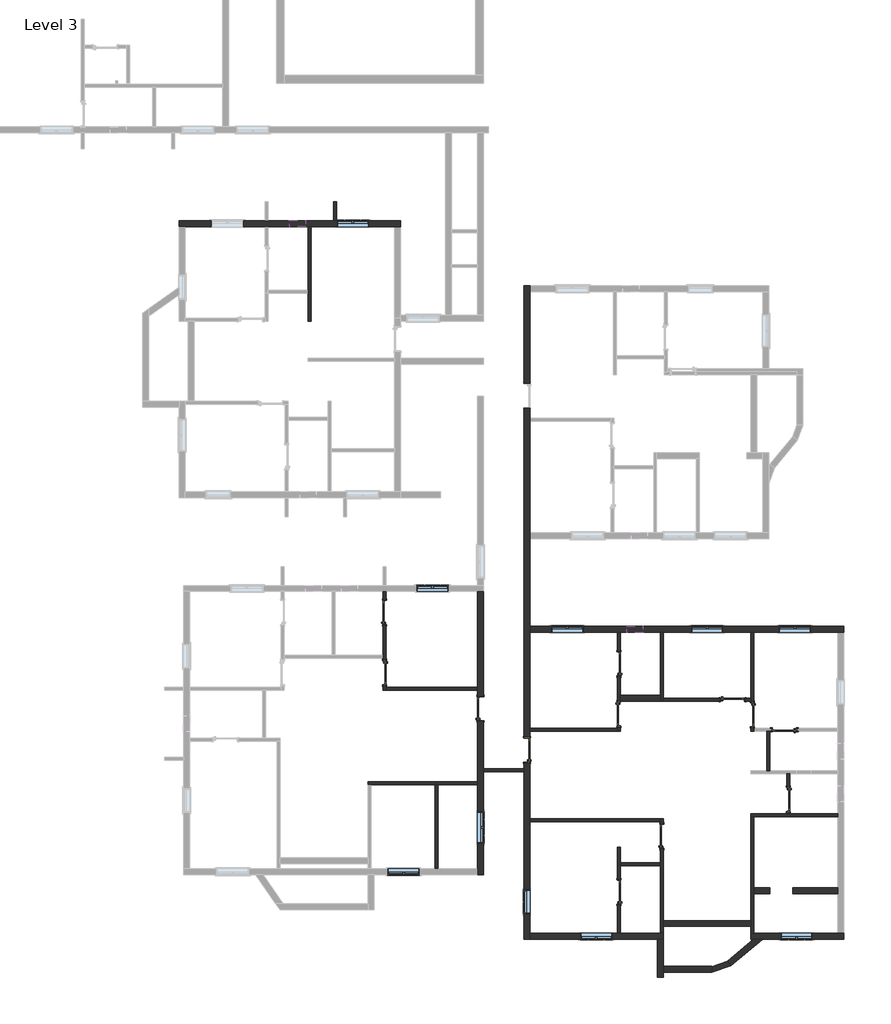
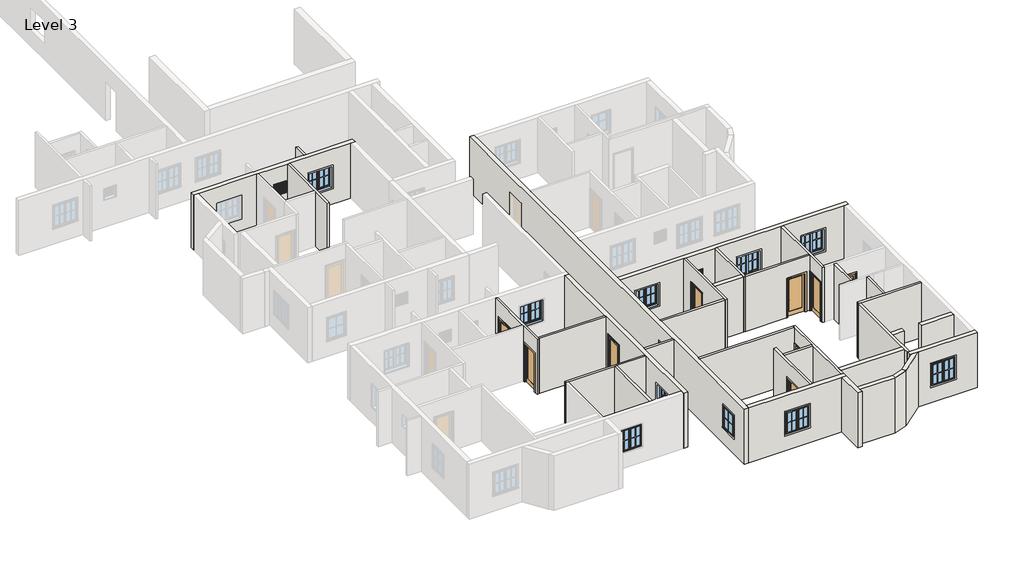
# One storey, part 2 of 7: 34 walls, 12 doors, 12 windows.
"""IFC4 building model written with IfcOpenShell, lengths in millimetres."""

from ifc_helpers import new_model, si_unit, frame, origin, place, context, project, spatial, polyline, circle_curve, outline, extrude, faceted_brep, transform, mapped, element, save
from ifc_brep_helpers import plane_surface, cylinder_surface, revolved_surface, advanced_brep
from components import door_3c6ab76a, door_a3feeac7, door_3b97b8e7, door_868ee8a9, window_272f20d6, window_casement_double_4_x_4_af3140d2, window_f2d8fef0

model = new_model("IFC4")

# Units and contexts
model_context = context("Model", 3, world=origin())
ifc_project = project(units=[si_unit("LENGTHUNIT", "METRE", prefix="MILLI")], contexts=[model_context])

# Site, building, storey
site = spatial("IfcSite", under=ifc_project)
building = spatial("IfcBuilding", under=site)
storey = spatial("IfcBuildingStorey", under=building, Name="Level 3", Elevation=3200.4)

# Doors
placement = place(None, origin())
door_shape = door_3c6ab76a(model_context)
element("IfcDoor", 1, ObjectType="Door-Interior-Single-1_Panel-Wood : 2'6\" x 7' door", at=placement, inside=storey, context=model_context, shape_type="MappedRepresentation", body=[
    mapped(door_shape, transform((13598.2490531, -20317.8247229, 3200.4), x_axis=(1.0, 0.0, 0.0), y_axis=(0.0, 1.0, 0.0), z_axis=(0.0, 0.0, 1.0))),
])
element("IfcDoor", 2, ObjectType="Door-Interior-Single-1_Panel-Wood : 2'6\" x 7' door", at=placement, inside=storey, context=model_context, shape_type="MappedRepresentation", body=[
    mapped(door_shape, transform((15579.4490531, -21467.1747229, 3200.4), x_axis=(-1.0, 0.0, 0.0), y_axis=(0.0, -1.0, 0.0), z_axis=(0.0, 0.0, 1.0))),
])
element("IfcDoor", 3, ObjectType="Door-Interior-Single-1_Panel-Wood : 2'6\" x 7' door", at=placement, inside=storey, context=model_context, shape_type="MappedRepresentation", body=[
    mapped(door_shape, transform((15735.0240531, -24130.9997229, 3200.4), x_axis=(0.0, -1.0, 0.0), y_axis=(1.0, 0.0, 0.0), z_axis=(0.0, 0.0, 1.0))),
])
element("IfcDoor", 4, ObjectType="Door-Interior-Single-1_Panel-Wood : 2'6\" x 7' door", at=placement, inside=storey, context=model_context, shape_type="MappedRepresentation", body=[
    mapped(door_shape, transform((285.4740531, -16985.9538828, 3200.4), x_axis=(0.0, 1.0, 0.0), y_axis=(-1.0, 0.0, 0.0), z_axis=(0.0, 0.0, 1.0))),
])
door_2_shape = door_a3feeac7(model_context)
element("IfcDoor", 5, ObjectType="Door-Interior-Single-1_Panel-Wood : 2'6\" x 7' door", at=placement, inside=storey, context=model_context, shape_type="MappedRepresentation", body=[
    mapped(door_2_shape, transform((9258.0240531, -18949.3997229, 3200.4), x_axis=(0.0, 1.0, 0.0), y_axis=(-1.0, 0.0, 0.0), z_axis=(0.0, 0.0, 1.0))),
])
element("IfcDoor", 6, ObjectType="Door-Interior-Single-1_Panel-Wood : 2'6\" x 7' door", at=placement, inside=storey, context=model_context, shape_type="MappedRepresentation", body=[
    mapped(door_2_shape, transform((9258.0240531, -27674.2997229, 3200.4), x_axis=(0.0, 1.0, 0.0), y_axis=(-1.0, 0.0, 0.0), z_axis=(0.0, 0.0, 1.0))),
])
element("IfcDoor", 7, ObjectType="Door-Interior-Single-1_Panel-Wood : 36\" x 84\"", at=placement, inside=storey, context=model_context, shape_type="MappedRepresentation", body=[
    mapped(door_shape, transform((14363.4240531, -20892.4997229, 3200.4), x_axis=(0.0, -1.0, 0.0), y_axis=(1.0, 0.0, 0.0), z_axis=(0.0, 0.0, 1.0))),
])
element("IfcDoor", 8, ObjectType="Door-Interior-Single-1_Panel-Wood : 36\" x 84\"", at=placement, inside=storey, context=model_context, shape_type="MappedRepresentation", body=[
    mapped(door_shape, transform((10889.9740531, -25540.6997229, 3200.4), x_axis=(0.0, 1.0, 0.0), y_axis=(-1.0, 0.0, 0.0), z_axis=(0.0, 0.0, 1.0))),
])
element("IfcDoor", 9, ObjectType="Door-Interior-Single-1_Panel-Wood : 36\" x 84\"", at=placement, inside=storey, context=model_context, shape_type="MappedRepresentation", body=[
    mapped(door_shape, transform((291.8240531, -19291.0038828, 3200.4), x_axis=(0.0, -1.0, 0.0), y_axis=(1.0, 0.0, 0.0), z_axis=(0.0, 0.0, 1.0))),
])
door_3_shape = door_3b97b8e7(model_context)
element("IfcDoor", 10, ObjectType="Door-Interior-Single-1_Panel-Wood : 36\" x 84\"", at=placement, inside=storey, context=model_context, shape_type="MappedRepresentation", body=[
    mapped(door_3_shape, transform((3962.1240531, -20662.6038828, 3200.4), x_axis=(0.0, 1.0, 0.0), y_axis=(-1.0, 0.0, 0.0), z_axis=(0.0, 0.0, 1.0))),
])
element("IfcDoor", 11, ObjectType="Door-Interior-Single-1_Panel-Wood : 36\" x 84\"", at=placement, inside=storey, context=model_context, shape_type="MappedRepresentation", body=[
    mapped(door_2_shape, transform((9251.6740531, -20863.9247229, 3200.4), x_axis=(0.0, -1.0, 0.0), y_axis=(1.0, 0.0, 0.0), z_axis=(0.0, 0.0, 1.0))),
])
door_4_shape = door_868ee8a9(model_context)
element("IfcDoor", 12, ObjectType="Door-Interior-Single-1_Panel-Wood : 36\" x 84\"", at=placement, inside=storey, context=model_context, shape_type="MappedRepresentation", body=[
    mapped(door_4_shape, transform((5733.7740531, -22245.3540434, 3200.4), x_axis=(0.0, 1.0, 0.0), y_axis=(-1.0, 0.0, 0.0), z_axis=(0.0, 0.0, 1.0))),
])

# Walls
element("IfcWall", 13, ObjectType="4.5\" wall", at=placement, inside=storey, context=model_context, shape_type="Brep", body=[
    faceted_brep([(-2524.4009469, -5860.7538828, 3200.4), (-2524.4009469, -2241.2538828, 3200.4), (-2524.4009469, -2241.2538828, 6248.4), (-2524.4009469, -5860.7538828, 6248.4), (-2638.7009469, -5860.7538828, 3200.4), (-2638.7009469, -5860.7538828, 6248.4), (-2638.7009469, -4793.9538828, 6248.4), (-2638.7009469, -4679.6538828, 6248.4), (-2638.7009469, -2241.2538828, 6248.4), (-2638.7009469, -2241.2538828, 3200.4), (-2638.7009469, -4679.6538828, 3200.4), (-2638.7009469, -4793.9538828, 3200.4)], [[[0, 1, 2, 3]], [[4, 5, 6, 7, 8, 9, 10, 11]], [[1, 0, 4, 11, 10, 9]], [[3, 2, 8, 7, 6, 5]], [[0, 3, 5, 4]], [[2, 1, 9, 8]]]),
])
element("IfcWall", 14, ObjectType="4.5\" wall", at=placement, inside=storey, context=model_context, shape_type="SweptSolid", body=[
    extrude(outline(polyline([(-1533.8009469, -1288.7538828), (-1533.8009469, -2012.6538828), (-1648.1009469, -2012.6538828), (-1648.1009469, -1288.7538828), (-1533.8009469, -1288.7538828)])), frame((0.0, 0.0, 3200.4), z_axis=(0.0, 0.0, 1.0), x_axis=(1.0, 0.0, 0.0)), (0.0, 0.0, 1.0), 3048.0),
])
element("IfcWall", 15, ObjectType="4.5\" wall", at=placement, inside=storey, context=model_context, shape_type="Brep", body=[
    faceted_brep([(345.7990531, -16185.8538828, 6248.4), (345.7990531, -19843.4538828, 6248.4), (345.7990531, -19957.7538828, 6248.4), (345.7990531, -19957.7538828, 3200.4), (345.7990531, -19843.4538828, 3200.4), (345.7990531, -19773.6038828, 3200.4), (345.7990531, -19773.6038828, 5359.4), (345.7990531, -18808.4038828, 5359.4), (345.7990531, -18808.4038828, 3200.4), (345.7990531, -17468.5538828, 3200.4), (345.7990531, -17468.5538828, 5359.4), (345.7990531, -16503.3538828, 5359.4), (345.7990531, -16503.3538828, 3200.4), (345.7990531, -16185.8538828, 3200.4), (231.4990531, -19957.7538828, 6248.4), (231.4990531, -18738.5538828, 6248.4), (231.4990531, -18624.2538828, 6248.4), (231.4990531, -16185.8538828, 6248.4), (231.4990531, -16185.8538828, 3200.4), (231.4990531, -16503.3538828, 3200.4), (231.4990531, -16503.3538828, 5359.4), (231.4990531, -17468.5538828, 5359.4), (231.4990531, -17468.5538828, 3200.4), (231.4990531, -18624.2538828, 3200.4), (231.4990531, -18738.5538828, 3200.4), (231.4990531, -18808.4038828, 3200.4), (231.4990531, -18808.4038828, 5359.4), (231.4990531, -19773.6038828, 5359.4), (231.4990531, -19773.6038828, 3200.4), (231.4990531, -19957.7538828, 3200.4)], [[[0, 1, 2, 3, 4, 5, 6, 7, 8, 9, 10, 11, 12, 13]], [[14, 15, 16, 17, 18, 19, 20, 21, 22, 23, 24, 25, 26, 27, 28, 29]], [[18, 13, 12, 19]], [[3, 29, 28, 5, 4]], [[22, 9, 8, 25, 24, 23]], [[2, 1, 0, 17, 16, 15, 14]], [[0, 13, 18, 17]], [[3, 2, 14, 29]], [[11, 20, 19, 12]], [[20, 11, 10, 21]], [[21, 10, 9, 22]], [[27, 6, 5, 28]], [[6, 27, 26, 7]], [[7, 26, 25, 8]]]),
])
element("IfcWall", 16, ObjectType="4.5\" wall", at=placement, inside=storey, context=model_context, shape_type="SweptSolid", body=[
    extrude(outline(polyline([(3850.9990531, -19957.7538828), (345.7990531, -19957.7538828), (345.7990531, -19843.4538828), (3850.9990531, -19843.4538828), (3850.9990531, -19957.7538828)])), frame((0.0, 0.0, 3200.4), z_axis=(0.0, 0.0, 1.0), x_axis=(1.0, 0.0, 0.0)), (0.0, 0.0, 1.0), 3048.0),
])
element("IfcWall", 17, ObjectType="4.5\" wall", at=placement, inside=storey, context=model_context, shape_type="Brep", body=[
    faceted_brep([(3850.9990531, -23462.9538828, 3200.4), (-340.0009469, -23462.9538828, 3200.4), (-340.0009469, -23462.9538828, 6248.4), (3850.9990531, -23462.9538828, 6248.4), (3850.9990531, -23577.2538828, 3200.4), (3850.9990531, -23577.2538828, 6248.4), (2326.9990531, -23577.2538828, 6248.4), (2212.6990531, -23577.2538828, 6248.4), (-225.7009469, -23577.2538828, 6248.4), (-340.0009469, -23577.2538828, 6248.4), (-340.0009469, -23577.2538828, 3200.4), (-225.7009469, -23577.2538828, 3200.4), (2212.6990531, -23577.2538828, 3200.4), (2326.9990531, -23577.2538828, 3200.4)], [[[0, 1, 2, 3]], [[4, 5, 6, 7, 8, 9, 10, 11, 12, 13]], [[1, 0, 4, 13, 12, 11, 10]], [[3, 2, 9, 8, 7, 6, 5]], [[0, 3, 5, 4]], [[2, 1, 10, 9]]]),
])
element("IfcWall", 18, ObjectType="4.5\" wall", at=placement, inside=storey, context=model_context, shape_type="SweptSolid", body=[
    extrude(outline(polyline([(2326.9990531, -23577.2538828), (2326.9990531, -26777.6538828), (2212.6990531, -26777.6538828), (2212.6990531, -23577.2538828), (2326.9990531, -23577.2538828)])), frame((0.0, 0.0, 3200.4), z_axis=(0.0, 0.0, 1.0), x_axis=(1.0, 0.0, 0.0)), (0.0, 0.0, 1.0), 3048.0),
])
element("IfcWall", 19, ObjectType="4.5\" wall", at=placement, inside=storey, context=model_context, shape_type="Brep", body=[
    faceted_brep([(10835.9990531, -17749.2497229, 3200.4), (10835.9990531, -20149.5497229, 3200.4), (10835.9990531, -20378.1497229, 3200.4), (10835.9990531, -20378.1497229, 6248.4), (10835.9990531, -20149.5497229, 6248.4), (10835.9990531, -17749.2497229, 6248.4), (10950.2990531, -17749.2497229, 3200.4), (10950.2990531, -17749.2497229, 6248.4), (10950.2990531, -20263.8497229, 6248.4), (10950.2990531, -20378.1497229, 6248.4), (10950.2990531, -20378.1497229, 3200.4), (10950.2990531, -20263.8497229, 3200.4)], [[[0, 1, 2, 3, 4, 5]], [[6, 7, 8, 9, 10, 11]], [[2, 1, 0, 6, 11, 10]], [[5, 4, 3, 9, 8, 7]], [[0, 5, 7, 6]], [[3, 2, 10, 9]]]),
])
element("IfcWall", 20, ObjectType="4.5\" wall", at=placement, inside=storey, context=model_context, shape_type="Brep", body=[
    faceted_brep([(9311.9990531, -17749.2497229, 6248.4), (9311.9990531, -20149.5497229, 6248.4), (9311.9990531, -20378.1497229, 6248.4), (9311.9990531, -21521.1497229, 6248.4), (9311.9990531, -21521.1497229, 3200.4), (9311.9990531, -21346.5247229, 3200.4), (9311.9990531, -21346.5247229, 5359.4), (9311.9990531, -20381.3247229, 5359.4), (9311.9990531, -20381.3247229, 3200.4), (9311.9990531, -20378.1497229, 3200.4), (9311.9990531, -20149.5497229, 3200.4), (9311.9990531, -19431.9997229, 3200.4), (9311.9990531, -19431.9997229, 5359.4), (9311.9990531, -18466.7997229, 5359.4), (9311.9990531, -18466.7997229, 3200.4), (9311.9990531, -17749.2497229, 3200.4), (9197.6990531, -21521.1497229, 6248.4), (9197.6990531, -21406.8497229, 6248.4), (9197.6990531, -17749.2497229, 6248.4), (9197.6990531, -17749.2497229, 3200.4), (9197.6990531, -18466.7997229, 3200.4), (9197.6990531, -18466.7997229, 5359.4), (9197.6990531, -19431.9997229, 5359.4), (9197.6990531, -19431.9997229, 3200.4), (9197.6990531, -20381.3247229, 3200.4), (9197.6990531, -20381.3247229, 5359.4), (9197.6990531, -21346.5247229, 5359.4), (9197.6990531, -21346.5247229, 3200.4), (9197.6990531, -21406.8497229, 3200.4), (9197.6990531, -21521.1497229, 3200.4)], [[[0, 1, 2, 3, 4, 5, 6, 7, 8, 9, 10, 11, 12, 13, 14, 15]], [[16, 17, 18, 19, 20, 21, 22, 23, 24, 25, 26, 27, 28, 29]], [[19, 15, 14, 20]], [[4, 29, 28, 27, 5]], [[8, 24, 23, 11, 10, 9]], [[3, 2, 1, 0, 18, 17, 16]], [[0, 15, 19, 18]], [[4, 3, 16, 29]], [[26, 6, 5, 27]], [[6, 26, 25, 7]], [[7, 25, 24, 8]], [[13, 21, 20, 14]], [[21, 13, 12, 22]], [[22, 12, 11, 23]]]),
])
element("IfcWall", 21, ObjectType="4.5\" wall", at=placement, inside=storey, context=model_context, shape_type="SweptSolid", body=[
    extrude(outline(polyline([(5844.8990531, -21406.8497229), (9197.6990531, -21406.8497229), (9197.6990531, -21521.1497229), (5844.8990531, -21521.1497229), (5844.8990531, -21406.8497229)])), frame((0.0, 0.0, 3200.4), z_axis=(0.0, 0.0, 1.0), x_axis=(1.0, 0.0, 0.0)), (0.0, 0.0, 1.0), 3048.0),
])
element("IfcWall", 22, ObjectType="4.5\" wall", at=placement, inside=storey, context=model_context, shape_type="Brep", body=[
    faceted_brep([(14303.0990531, -21521.1497229, 6248.4), (14303.0990531, -20378.1497229, 6248.4), (14303.0990531, -20263.8497229, 6248.4), (14303.0990531, -17749.2497229, 6248.4), (14303.0990531, -17749.2497229, 3200.4), (14303.0990531, -20263.8497229, 3200.4), (14303.0990531, -20378.1497229, 3200.4), (14303.0990531, -20409.8997229, 3200.4), (14303.0990531, -20409.8997229, 5359.4), (14303.0990531, -21375.0997229, 5359.4), (14303.0990531, -21375.0997229, 3200.4), (14303.0990531, -21521.1497229, 3200.4), (14417.3990531, -17749.2497229, 6248.4), (14417.3990531, -21406.8497229, 6248.4), (14417.3990531, -21521.1497229, 6248.4), (14417.3990531, -21521.1497229, 3200.4), (14417.3990531, -21406.8497229, 3200.4), (14417.3990531, -21375.0997229, 3200.4), (14417.3990531, -21375.0997229, 5359.4), (14417.3990531, -20409.8997229, 5359.4), (14417.3990531, -20409.8997229, 3200.4), (14417.3990531, -17749.2497229, 3200.4)], [[[0, 1, 2, 3, 4, 5, 6, 7, 8, 9, 10, 11]], [[12, 13, 14, 15, 16, 17, 18, 19, 20, 21]], [[4, 21, 20, 7, 6, 5]], [[15, 11, 10, 17, 16]], [[3, 2, 1, 0, 14, 13, 12]], [[4, 3, 12, 21]], [[0, 11, 15, 14]], [[9, 18, 17, 10]], [[18, 9, 8, 19]], [[19, 8, 7, 20]]]),
])
element("IfcWall", 23, ObjectType="4.5\" wall", at=placement, inside=storey, context=model_context, shape_type="Brep", body=[
    faceted_brep([(14303.0990531, -24797.7497229, 3200.4), (14417.3990531, -24797.7497229, 3200.4), (17617.7990531, -24797.7497229, 3200.4), (17617.7990531, -24797.7497229, 6248.4), (14417.3990531, -24797.7497229, 6248.4), (14303.0990531, -24797.7497229, 6248.4), (14303.0990531, -24683.4497229, 3200.4), (14303.0990531, -24683.4497229, 6248.4), (15674.6990531, -24683.4497229, 6248.4), (15788.9990531, -24683.4497229, 6248.4), (17617.7990531, -24683.4497229, 6248.4), (17617.7990531, -24683.4497229, 3200.4), (15788.9990531, -24683.4497229, 3200.4), (15674.6990531, -24683.4497229, 3200.4)], [[[0, 1, 2, 3, 4, 5]], [[6, 7, 8, 9, 10, 11, 12, 13]], [[2, 1, 0, 6, 13, 12, 11]], [[5, 4, 3, 10, 9, 8, 7]], [[3, 2, 11, 10]], [[0, 5, 7, 6]]]),
])
element("IfcWall", 24, ObjectType="4.5\" wall", at=placement, inside=storey, context=model_context, shape_type="Brep", body=[
    faceted_brep([(14417.3990531, -29255.4497229, 3200.4), (14417.3990531, -27731.4497229, 3200.4), (14417.3990531, -27502.8497229, 3200.4), (14417.3990531, -24797.7497229, 3200.4), (14417.3990531, -24797.7497229, 6248.4), (14417.3990531, -27502.8497229, 6248.4), (14417.3990531, -27731.4497229, 6248.4), (14417.3990531, -29255.4497229, 6248.4), (14303.0990531, -29255.4497229, 3200.4), (14303.0990531, -29255.4497229, 6248.4), (14303.0990531, -28988.7497229, 6248.4), (14303.0990531, -28760.1497229, 6248.4), (14303.0990531, -24797.7497229, 6248.4), (14303.0990531, -24797.7497229, 3200.4), (14303.0990531, -28760.1497229, 3200.4), (14303.0990531, -28988.7497229, 3200.4)], [[[0, 1, 2, 3, 4, 5, 6, 7]], [[8, 9, 10, 11, 12, 13, 14, 15]], [[3, 2, 1, 0, 8, 15, 14, 13]], [[7, 6, 5, 4, 12, 11, 10, 9]], [[4, 3, 13, 12]], [[0, 7, 9, 8]]]),
])
element("IfcWall", 25, ObjectType="4.5\" wall", at=placement, inside=storey, context=model_context, shape_type="SweptSolid", body=[
    extrude(outline(polyline([(6248.4, 14303.0990531), (6248.4, 10950.2990531), (3200.4, 10950.2990531), (3200.4, 13115.6490531), (5359.4, 13115.6490531), (5359.4, 14080.8490531), (3200.4, 14080.8490531), (3200.4, 14303.0990531), (6248.4, 14303.0990531)])), frame((0.0, -20378.1497229, 0.0), z_axis=(0.0, 1.0, 0.0), x_axis=(0.0, 0.0, 1.0)), (0.0, 0.0, 1.0), 114.3),
])
element("IfcWall", 26, ObjectType="4.5\" wall", at=placement, inside=storey, context=model_context, shape_type="SweptSolid", body=[
    extrude(outline(polyline([(14912.6990531, -23045.1497229), (14912.6990531, -21521.1497229), (15026.9990531, -21521.1497229), (15026.9990531, -23045.1497229), (14912.6990531, -23045.1497229)])), frame((0.0, 0.0, 3200.4), z_axis=(0.0, 0.0, 1.0), x_axis=(1.0, 0.0, 0.0)), (0.0, 0.0, 1.0), 3048.0),
])
element("IfcWall", 27, ObjectType="4.5\" wall", at=placement, inside=storey, context=model_context, shape_type="Brep", body=[
    faceted_brep([(10835.9990531, -29255.4497229, 6248.4), (10835.9990531, -26664.6497229, 6248.4), (10835.9990531, -26550.3497229, 6248.4), (10835.9990531, -24988.2497229, 6248.4), (10835.9990531, -24873.9497229, 6248.4), (10835.9990531, -24873.9497229, 3200.4), (10835.9990531, -24988.2497229, 3200.4), (10835.9990531, -25058.0997229, 3200.4), (10835.9990531, -25058.0997229, 5359.4), (10835.9990531, -26023.2997229, 5359.4), (10835.9990531, -26023.2997229, 3200.4), (10835.9990531, -26550.3497229, 3200.4), (10835.9990531, -26664.6497229, 3200.4), (10835.9990531, -29255.4497229, 3200.4), (10950.2990531, -24873.9497229, 6248.4), (10950.2990531, -28760.1497229, 6248.4), (10950.2990531, -28988.7497229, 6248.4), (10950.2990531, -29255.4497229, 6248.4), (10950.2990531, -29255.4497229, 3200.4), (10950.2990531, -28988.7497229, 3200.4), (10950.2990531, -28760.1497229, 3200.4), (10950.2990531, -26023.2997229, 3200.4), (10950.2990531, -26023.2997229, 5359.4), (10950.2990531, -25058.0997229, 5359.4), (10950.2990531, -25058.0997229, 3200.4), (10950.2990531, -24873.9497229, 3200.4)], [[[0, 1, 2, 3, 4, 5, 6, 7, 8, 9, 10, 11, 12, 13]], [[14, 15, 16, 17, 18, 19, 20, 21, 22, 23, 24, 25]], [[18, 13, 12, 11, 10, 21, 20, 19]], [[5, 25, 24, 7, 6]], [[4, 3, 2, 1, 0, 17, 16, 15, 14]], [[0, 13, 18, 17]], [[5, 4, 14, 25]], [[23, 8, 7, 24]], [[8, 23, 22, 9]], [[9, 22, 21, 10]]]),
])
element("IfcWall", 28, ObjectType="4.5\" wall", at=placement, inside=storey, context=model_context, shape_type="SweptSolid", body=[
    extrude(outline(polyline([(10835.9990531, -24988.2497229), (5844.8990531, -24988.2497229), (5844.8990531, -24873.9497229), (10835.9990531, -24873.9497229), (10835.9990531, -24988.2497229)])), frame((0.0, 0.0, 3200.4), z_axis=(0.0, 0.0, 1.0), x_axis=(1.0, 0.0, 0.0)), (0.0, 0.0, 1.0), 3048.0),
])
element("IfcWall", 29, ObjectType="4.5\" wall", at=placement, inside=storey, context=model_context, shape_type="SweptSolid", body=[
    extrude(outline(polyline([(-24683.4497229, 6248.4), (-23159.4497229, 6248.4), (-23159.4497229, 3200.4), (-23648.3997229, 3200.4), (-23648.3997229, 5359.4), (-24613.5997229, 5359.4), (-24613.5997229, 3200.4), (-24683.4497229, 3200.4), (-24683.4497229, 6248.4)])), frame((15674.6990531, 0.0, 0.0), z_axis=(1.0, 0.0, 0.0), x_axis=(0.0, 1.0, 0.0)), (0.0, 0.0, 1.0), 114.3),
])
element("IfcWall", 30, ObjectType="4.5\" wall", at=placement, inside=storey, context=model_context, shape_type="SweptSolid", body=[
    extrude(outline(polyline([(10835.9990531, -26664.6497229), (9311.9990531, -26664.6497229), (9311.9990531, -26550.3497229), (10835.9990531, -26550.3497229), (10835.9990531, -26664.6497229)])), frame((0.0, 0.0, 3200.4), z_axis=(0.0, 0.0, 1.0), x_axis=(1.0, 0.0, 0.0)), (0.0, 0.0, 1.0), 3048.0),
])
element("IfcWall", 31, ObjectType="4.5\" wall", at=placement, inside=storey, context=model_context, shape_type="Brep", body=[
    faceted_brep([(9311.9990531, -25953.4497229, 3200.4), (9311.9990531, -25953.4497229, 6248.4), (9311.9990531, -26550.3497229, 6248.4), (9311.9990531, -26664.6497229, 6248.4), (9311.9990531, -29255.4497229, 6248.4), (9311.9990531, -29255.4497229, 3200.4), (9311.9990531, -28156.8997229, 3200.4), (9311.9990531, -28156.8997229, 5359.4), (9311.9990531, -27191.6997229, 5359.4), (9311.9990531, -27191.6997229, 3200.4), (9311.9990531, -26664.6497229, 3200.4), (9311.9990531, -26550.3497229, 3200.4), (9197.6990531, -25953.4497229, 6248.4), (9197.6990531, -25953.4497229, 3200.4), (9197.6990531, -27191.6997229, 3200.4), (9197.6990531, -27191.6997229, 5359.4), (9197.6990531, -28156.8997229, 5359.4), (9197.6990531, -28156.8997229, 3200.4), (9197.6990531, -29255.4497229, 3200.4), (9197.6990531, -29255.4497229, 6248.4)], [[[0, 1, 2, 3, 4, 5, 6, 7, 8, 9, 10, 11]], [[12, 13, 14, 15, 16, 17, 18, 19]], [[13, 0, 11, 10, 9, 14]], [[5, 18, 17, 6]], [[1, 0, 13, 12]], [[4, 3, 2, 1, 12, 19]], [[5, 4, 19, 18]], [[8, 15, 14, 9]], [[15, 8, 7, 16]], [[16, 7, 6, 17]]]),
])
element("IfcWall", 32, ObjectType="4.5\" wall", at=placement, inside=storey, context=model_context, shape_type="SweptSolid", body=[
    extrude(outline(polyline([(4079.5990531, -22969.5583639), (5616.2990531, -22969.5583639), (5616.2990531, -23083.8583639), (4079.5990531, -23083.8583639), (4079.5990531, -22969.5583639)])), frame((0.0, 0.0, 3200.4), z_axis=(0.0, 0.0, 1.0), x_axis=(1.0, 0.0, 0.0)), (0.0, 0.0, 1.0), 3048.0),
])
element("IfcWall", 33, ObjectType="9\"", at=placement, inside=storey, context=model_context, shape_type="Brep", body=[
    faceted_brep([(904.5990531, -2012.6538828, 3200.4), (-1533.8009469, -2012.6538828, 3200.4), (-1648.1009469, -2012.6538828, 3200.4), (-4162.7009469, -2012.6538828, 3200.4), (-4277.0009469, -2012.6538828, 3200.4), (-7553.6009469, -2012.6538828, 3200.4), (-7553.6009469, -2012.6538828, 6248.4), (-4277.0009469, -2012.6538828, 6248.4), (-4162.7009469, -2012.6538828, 6248.4), (-1648.1009469, -2012.6538828, 6248.4), (-1533.8009469, -2012.6538828, 6248.4), (904.5990531, -2012.6538828, 6248.4), (-2733.9509469, -2012.6538828, 5334.0), (-3343.5509469, -2012.6538828, 5334.0), (-3343.5509469, -2012.6538828, 4724.4), (-2733.9509469, -2012.6538828, 4724.4), (-5108.8509469, -2012.6538828, 5334.0), (-6328.0509469, -2012.6538828, 5334.0), (-6328.0509469, -2012.6538828, 4114.8), (-5108.8509469, -2012.6538828, 4114.8), (-308.2509469, -2012.6538828, 5334.0), (-1527.4509469, -2012.6538828, 5334.0), (-1527.4509469, -2012.6538828, 4114.8), (-308.2509469, -2012.6538828, 4114.8), (904.5990531, -2241.2538828, 3200.4), (904.5990531, -2241.2538828, 6248.4), (675.9990531, -2241.2538828, 6248.4), (-2524.4009469, -2241.2538828, 6248.4), (-2638.7009469, -2241.2538828, 6248.4), (-4162.7009469, -2241.2538828, 6248.4), (-4277.0009469, -2241.2538828, 6248.4), (-7325.0009469, -2241.2538828, 6248.4), (-7553.6009469, -2241.2538828, 6248.4), (-7553.6009469, -2241.2538828, 3200.4), (-7325.0009469, -2241.2538828, 3200.4), (-4277.0009469, -2241.2538828, 3200.4), (-4162.7009469, -2241.2538828, 3200.4), (-2638.7009469, -2241.2538828, 3200.4), (-2524.4009469, -2241.2538828, 3200.4), (675.9990531, -2241.2538828, 3200.4), (-2733.9509469, -2241.2538828, 5334.0), (-2733.9509469, -2241.2538828, 4724.4), (-3343.5509469, -2241.2538828, 4724.4), (-3343.5509469, -2241.2538828, 5334.0), (-5108.8509469, -2241.2538828, 5334.0), (-5108.8509469, -2241.2538828, 4114.8), (-6328.0509469, -2241.2538828, 4114.8), (-6328.0509469, -2241.2538828, 5334.0), (-308.2509469, -2241.2538828, 5334.0), (-308.2509469, -2241.2538828, 4114.8), (-1527.4509469, -2241.2538828, 4114.8), (-1527.4509469, -2241.2538828, 5334.0)], [[[0, 1, 2, 3, 4, 5, 6, 7, 8, 9, 10, 11], [12, 13, 14, 15], [16, 17, 18, 19], [20, 21, 22, 23]], [[24, 25, 26, 27, 28, 29, 30, 31, 32, 33, 34, 35, 36, 37, 38, 39], [40, 41, 42, 43], [44, 45, 46, 47], [48, 49, 50, 51]], [[5, 4, 3, 2, 1, 0, 24, 39, 38, 37, 36, 35, 34, 33]], [[11, 10, 9, 8, 7, 6, 32, 31, 30, 29, 28, 27, 26, 25]], [[0, 11, 25, 24]], [[6, 5, 33, 32]], [[41, 40, 12, 15]], [[42, 41, 15, 14]], [[43, 42, 14, 13]], [[40, 43, 13, 12]], [[45, 44, 16, 19]], [[46, 45, 19, 18]], [[47, 46, 18, 17]], [[44, 47, 17, 16]], [[49, 48, 20, 23]], [[50, 49, 23, 22]], [[51, 50, 22, 21]], [[48, 51, 21, 20]]]),
])
element("IfcWall", 34, ObjectType="9\"", at=placement, inside=storey, context=model_context, shape_type="Brep", body=[
    faceted_brep([(4079.5990531, -16185.8538828, 6248.4), (4079.5990531, -22969.5583639, 6248.4), (4079.5990531, -23083.8583639, 6248.4), (4079.5990531, -27006.2538828, 6248.4), (4079.5990531, -27006.2538828, 3200.4), (4079.5990531, -23083.8583639, 3200.4), (4079.5990531, -22969.5583639, 3200.4), (4079.5990531, -21145.2038828, 3200.4), (4079.5990531, -21145.2038828, 5359.4), (4079.5990531, -20180.0038828, 5359.4), (4079.5990531, -20180.0038828, 3200.4), (4079.5990531, -16185.8538828, 3200.4), (4079.5990531, -25815.6288828, 5334.0), (4079.5990531, -24596.4288828, 5334.0), (4079.5990531, -24596.4288828, 4114.8), (4079.5990531, -25815.6288828, 4114.8), (3850.9990531, -27006.2538828, 6248.4), (3850.9990531, -26777.6538828, 6248.4), (3850.9990531, -23577.2538828, 6248.4), (3850.9990531, -23462.9538828, 6248.4), (3850.9990531, -19957.7538828, 6248.4), (3850.9990531, -19843.4538828, 6248.4), (3850.9990531, -16185.8538828, 6248.4), (3850.9990531, -16185.8538828, 3200.4), (3850.9990531, -19843.4538828, 3200.4), (3850.9990531, -19957.7538828, 3200.4), (3850.9990531, -20180.0038828, 3200.4), (3850.9990531, -20180.0038828, 5359.4), (3850.9990531, -21145.2038828, 5359.4), (3850.9990531, -21145.2038828, 3200.4), (3850.9990531, -23462.9538828, 3200.4), (3850.9990531, -23577.2538828, 3200.4), (3850.9990531, -26777.6538828, 3200.4), (3850.9990531, -27006.2538828, 3200.4), (3850.9990531, -25815.6288828, 5334.0), (3850.9990531, -25815.6288828, 4114.8), (3850.9990531, -24596.4288828, 4114.8), (3850.9990531, -24596.4288828, 5334.0)], [[[0, 1, 2, 3, 4, 5, 6, 7, 8, 9, 10, 11], [12, 13, 14, 15]], [[16, 17, 18, 19, 20, 21, 22, 23, 24, 25, 26, 27, 28, 29, 30, 31, 32, 33], [34, 35, 36, 37]], [[4, 33, 32, 31, 30, 29, 7, 6, 5]], [[23, 11, 10, 26, 25, 24]], [[3, 2, 1, 0, 22, 21, 20, 19, 18, 17, 16]], [[4, 3, 16, 33]], [[0, 11, 23, 22]], [[9, 27, 26, 10]], [[27, 9, 8, 28]], [[28, 8, 7, 29]], [[35, 34, 12, 15]], [[36, 35, 15, 14]], [[37, 36, 14, 13]], [[34, 37, 13, 12]]]),
])
element("IfcWall", 35, ObjectType="9\"", at=placement, inside=storey, context=model_context, shape_type="Brep", body=[
    faceted_brep([(5844.8990531, -17749.2497229, 3200.4), (9197.6990531, -17749.2497229, 3200.4), (9311.9990531, -17749.2497229, 3200.4), (10835.9990531, -17749.2497229, 3200.4), (10950.2990531, -17749.2497229, 3200.4), (14303.0990531, -17749.2497229, 3200.4), (14417.3990531, -17749.2497229, 3200.4), (17617.7990531, -17749.2497229, 3200.4), (17846.3990531, -17749.2497229, 3200.4), (17846.3990531, -17749.2497229, 6248.4), (17617.7990531, -17749.2497229, 6248.4), (14417.3990531, -17749.2497229, 6248.4), (14303.0990531, -17749.2497229, 6248.4), (10950.2990531, -17749.2497229, 6248.4), (10835.9990531, -17749.2497229, 6248.4), (9311.9990531, -17749.2497229, 6248.4), (9197.6990531, -17749.2497229, 6248.4), (5844.8990531, -17749.2497229, 6248.4), (10169.2490531, -17749.2497229, 5334.0), (10169.2490531, -17749.2497229, 4724.4), (9559.6490531, -17749.2497229, 4724.4), (9559.6490531, -17749.2497229, 5334.0), (7889.5990531, -17749.2497229, 5334.0), (7889.5990531, -17749.2497229, 4114.8), (6670.3990531, -17749.2497229, 4114.8), (6670.3990531, -17749.2497229, 5334.0), (13236.2990531, -17749.2497229, 5334.0), (13236.2990531, -17749.2497229, 4114.8), (12017.0990531, -17749.2497229, 4114.8), (12017.0990531, -17749.2497229, 5334.0), (16595.4490531, -17749.2497229, 5334.0), (16595.4490531, -17749.2497229, 4114.8), (15376.2490531, -17749.2497229, 4114.8), (15376.2490531, -17749.2497229, 5334.0), (5844.8990531, -17520.6497229, 3200.4), (5844.8990531, -17520.6497229, 6248.4), (17846.3990531, -17520.6497229, 6248.4), (17846.3990531, -17520.6497229, 3200.4), (10169.2490531, -17520.6497229, 5334.0), (9559.6490531, -17520.6497229, 5334.0), (9559.6490531, -17520.6497229, 4724.4), (10169.2490531, -17520.6497229, 4724.4), (7889.5990531, -17520.6497229, 5334.0), (6670.3990531, -17520.6497229, 5334.0), (6670.3990531, -17520.6497229, 4114.8), (7889.5990531, -17520.6497229, 4114.8), (13236.2990531, -17520.6497229, 5334.0), (12017.0990531, -17520.6497229, 5334.0), (12017.0990531, -17520.6497229, 4114.8), (13236.2990531, -17520.6497229, 4114.8), (16595.4490531, -17520.6497229, 5334.0), (15376.2490531, -17520.6497229, 5334.0), (15376.2490531, -17520.6497229, 4114.8), (16595.4490531, -17520.6497229, 4114.8)], [[[0, 1, 2, 3, 4, 5, 6, 7, 8, 9, 10, 11, 12, 13, 14, 15, 16, 17], [18, 19, 20, 21], [22, 23, 24, 25], [26, 27, 28, 29], [30, 31, 32, 33]], [[34, 35, 36, 37], [38, 39, 40, 41], [42, 43, 44, 45], [46, 47, 48, 49], [50, 51, 52, 53]], [[8, 7, 6, 5, 4, 3, 2, 1, 0, 34, 37]], [[17, 16, 15, 14, 13, 12, 11, 10, 9, 36, 35]], [[0, 17, 35, 34]], [[9, 8, 37, 36]], [[19, 18, 38, 41]], [[20, 19, 41, 40]], [[21, 20, 40, 39]], [[18, 21, 39, 38]], [[23, 22, 42, 45]], [[24, 23, 45, 44]], [[25, 24, 44, 43]], [[22, 25, 43, 42]], [[27, 26, 46, 49]], [[28, 27, 49, 48]], [[29, 28, 48, 47]], [[26, 29, 47, 46]], [[31, 30, 50, 53]], [[32, 31, 53, 52]], [[33, 32, 52, 51]], [[30, 33, 51, 50]]]),
])
element("IfcWall", 36, ObjectType="9\"", at=placement, inside=storey, context=model_context, shape_type="Brep", body=[
    faceted_brep([(5844.8990531, -4503.1497229, 6248.4), (5844.8990531, -4731.7497229, 6248.4), (5844.8990531, -9557.7497229, 6248.4), (5844.8990531, -9672.0497229, 6248.4), (5844.8990531, -13939.2497229, 6248.4), (5844.8990531, -14167.8497229, 6248.4), (5844.8990531, -17520.6497229, 6248.4), (5844.8990531, -17749.2497229, 6248.4), (5844.8990531, -21406.8497229, 6248.4), (5844.8990531, -21521.1497229, 6248.4), (5844.8990531, -24873.9497229, 6248.4), (5844.8990531, -24988.2497229, 6248.4), (5844.8990531, -29255.4497229, 6248.4), (5844.8990531, -29484.0497229, 6248.4), (5844.8990531, -29484.0497229, 3200.4), (5844.8990531, -29255.4497229, 3200.4), (5844.8990531, -24988.2497229, 3200.4), (5844.8990531, -24873.9497229, 3200.4), (5844.8990531, -22727.9540434, 3200.4), (5844.8990531, -22727.9540434, 5359.4), (5844.8990531, -21762.7540434, 5359.4), (5844.8990531, -21762.7540434, 3200.4), (5844.8990531, -21521.1497229, 3200.4), (5844.8990531, -21406.8497229, 3200.4), (5844.8990531, -17749.2497229, 3200.4), (5844.8990531, -17520.6497229, 3200.4), (5844.8990531, -14167.8497229, 3200.4), (5844.8990531, -13939.2497229, 3200.4), (5844.8990531, -9672.0497229, 3200.4), (5844.8990531, -9557.7497229, 3200.4), (5844.8990531, -9183.0997229, 3200.4), (5844.8990531, -9183.0997229, 5359.4), (5844.8990531, -8217.8997229, 5359.4), (5844.8990531, -8217.8997229, 3200.4), (5844.8990531, -4731.7497229, 3200.4), (5844.8990531, -4503.1497229, 3200.4), (5844.8990531, -27591.7497229, 5334.0), (5844.8990531, -27591.7497229, 4114.8), (5844.8990531, -28506.1497229, 4114.8), (5844.8990531, -28506.1497229, 5334.0), (5616.2990531, -29484.0497229, 6248.4), (5616.2990531, -23083.8583639, 6248.4), (5616.2990531, -22969.5583639, 6248.4), (5616.2990531, -4503.1497229, 6248.4), (5616.2990531, -4503.1497229, 3200.4), (5616.2990531, -8217.8997229, 3200.4), (5616.2990531, -8217.8997229, 5359.4), (5616.2990531, -9183.0997229, 5359.4), (5616.2990531, -9183.0997229, 3200.4), (5616.2990531, -21762.7540434, 3200.4), (5616.2990531, -21762.7540434, 5359.4), (5616.2990531, -22727.9540434, 5359.4), (5616.2990531, -22727.9540434, 3200.4), (5616.2990531, -22969.5583639, 3200.4), (5616.2990531, -23083.8583639, 3200.4), (5616.2990531, -29484.0497229, 3200.4), (5616.2990531, -27591.7497229, 5334.0), (5616.2990531, -28506.1497229, 5334.0), (5616.2990531, -28506.1497229, 4114.8), (5616.2990531, -27591.7497229, 4114.8)], [[[0, 1, 2, 3, 4, 5, 6, 7, 8, 9, 10, 11, 12, 13, 14, 15, 16, 17, 18, 19, 20, 21, 22, 23, 24, 25, 26, 27, 28, 29, 30, 31, 32, 33, 34, 35], [36, 37, 38, 39]], [[40, 41, 42, 43, 44, 45, 46, 47, 48, 49, 50, 51, 52, 53, 54, 55], [56, 57, 58, 59]], [[14, 55, 54, 53, 52, 18, 17, 16, 15]], [[44, 35, 34, 33, 45]], [[48, 30, 29, 28, 27, 26, 25, 24, 23, 22, 21, 49]], [[13, 12, 11, 10, 9, 8, 7, 6, 5, 4, 3, 2, 1, 0, 43, 42, 41, 40]], [[14, 13, 40, 55]], [[0, 35, 44, 43]], [[47, 31, 30, 48]], [[31, 47, 46, 32]], [[32, 46, 45, 33]], [[20, 50, 49, 21]], [[50, 20, 19, 51]], [[51, 19, 18, 52]], [[37, 36, 56, 59]], [[38, 37, 59, 58]], [[39, 38, 58, 57]], [[36, 39, 57, 56]]]),
])
element("IfcWall", 37, ObjectType="9\"", at=placement, inside=storey, context=model_context, shape_type="Brep", body=[
    faceted_brep([(5844.8990531, -29484.0497229, 3200.4), (10721.6990531, -29484.0497229, 3200.4), (10950.2990531, -29484.0497229, 3200.4), (10950.2990531, -29484.0497229, 6248.4), (10721.6990531, -29484.0497229, 6248.4), (5844.8990531, -29484.0497229, 6248.4), (7781.6490531, -29484.0497229, 5334.0), (9000.8490531, -29484.0497229, 5334.0), (9000.8490531, -29484.0497229, 4114.8), (7781.6490531, -29484.0497229, 4114.8), (5844.8990531, -29255.4497229, 3200.4), (5844.8990531, -29255.4497229, 6248.4), (9197.6990531, -29255.4497229, 6248.4), (9311.9990531, -29255.4497229, 6248.4), (10835.9990531, -29255.4497229, 6248.4), (10950.2990531, -29255.4497229, 6248.4), (10950.2990531, -29255.4497229, 3200.4), (10835.9990531, -29255.4497229, 3200.4), (9311.9990531, -29255.4497229, 3200.4), (9197.6990531, -29255.4497229, 3200.4), (7781.6490531, -29255.4497229, 5334.0), (7781.6490531, -29255.4497229, 4114.8), (9000.8490531, -29255.4497229, 4114.8), (9000.8490531, -29255.4497229, 5334.0)], [[[0, 1, 2, 3, 4, 5], [6, 7, 8, 9]], [[10, 11, 12, 13, 14, 15, 16, 17, 18, 19], [20, 21, 22, 23]], [[2, 1, 0, 10, 19, 18, 17, 16]], [[5, 4, 3, 15, 14, 13, 12, 11]], [[0, 5, 11, 10]], [[3, 2, 16, 15]], [[21, 20, 6, 9]], [[22, 21, 9, 8]], [[23, 22, 8, 7]], [[20, 23, 7, 6]]]),
])
element("IfcWall", 38, ObjectType="9\"", at=placement, inside=storey, context=model_context, shape_type="SweptSolid", body=[
    extrude(outline(polyline([(9311.9990531, -20149.5497229), (10835.9990531, -20149.5497229), (10835.9990531, -20378.1497229), (9311.9990531, -20378.1497229), (9311.9990531, -20149.5497229)])), frame((0.0, 0.0, 3200.4), z_axis=(0.0, 0.0, 1.0), x_axis=(1.0, 0.0, 0.0)), (0.0, 0.0, 1.0), 3048.0),
])
element("IfcWall", 39, ObjectType="9\"", at=placement, inside=storey, context=model_context, shape_type="SweptSolid", body=[
    extrude(outline(polyline([(17617.7990531, -27731.4497229), (15901.9350228, -27731.4497229), (15901.9350228, -27502.8497229), (17617.7990531, -27502.8497229), (17617.7990531, -27731.4497229)])), frame((0.0, 0.0, 3200.4), z_axis=(0.0, 0.0, 1.0), x_axis=(1.0, 0.0, 0.0)), (0.0, 0.0, 1.0), 3048.0),
])
element("IfcWall", 40, ObjectType="9\"", at=placement, inside=storey, context=model_context, shape_type="SweptSolid", body=[
    extrude(outline(polyline([(15026.9990531, -27731.4497229), (14417.3990531, -27731.4497229), (14417.3990531, -27502.8497229), (15026.9990531, -27502.8497229), (15026.9990531, -27731.4497229)])), frame((0.0, 0.0, 3200.4), z_axis=(0.0, 0.0, 1.0), x_axis=(1.0, 0.0, 0.0)), (0.0, 0.0, 1.0), 3048.0),
])
element("IfcWall", 41, ObjectType="9\"", at=placement, inside=storey, context=model_context, shape_type="SweptSolid", body=[
    extrude(outline(polyline([(14303.0990531, -28988.7497229), (10950.2990531, -28988.7497229), (10950.2990531, -28760.1497229), (14303.0990531, -28760.1497229), (14303.0990531, -28988.7497229)])), frame((0.0, 0.0, 3200.4), z_axis=(0.0, 0.0, 1.0), x_axis=(1.0, 0.0, 0.0)), (0.0, 0.0, 1.0), 3048.0),
])
element("IfcWall", 42, ObjectType="9\"", at=placement, inside=storey, context=model_context, shape_type="Brep", body=[
    faceted_brep([(14303.0990531, -29484.0497229, 3200.4), (14391.7049387, -29484.0497229, 3200.4), (14750.9761043, -29484.0497229, 3200.4), (17846.3990531, -29484.0497229, 3200.4), (17846.3990531, -29484.0497229, 6248.4), (14750.9761043, -29484.0497229, 6248.4), (14391.7049387, -29484.0497229, 6248.4), (14303.0990531, -29484.0497229, 6248.4), (15436.5740531, -29484.0497229, 5334.0), (16655.7740531, -29484.0497229, 5334.0), (16655.7740531, -29484.0497229, 4114.8), (15436.5740531, -29484.0497229, 4114.8), (14303.0990531, -29255.4497229, 3200.4), (14303.0990531, -29255.4497229, 6248.4), (14417.3990531, -29255.4497229, 6248.4), (17617.7990531, -29255.4497229, 6248.4), (17846.3990531, -29255.4497229, 6248.4), (17846.3990531, -29255.4497229, 3200.4), (17617.7990531, -29255.4497229, 3200.4), (14417.3990531, -29255.4497229, 3200.4), (15436.5740531, -29255.4497229, 5334.0), (15436.5740531, -29255.4497229, 4114.8), (16655.7740531, -29255.4497229, 4114.8), (16655.7740531, -29255.4497229, 5334.0)], [[[0, 1, 2, 3, 4, 5, 6, 7], [8, 9, 10, 11]], [[12, 13, 14, 15, 16, 17, 18, 19], [20, 21, 22, 23]], [[3, 2, 1, 0, 12, 19, 18, 17]], [[7, 6, 5, 4, 16, 15, 14, 13]], [[4, 3, 17, 16]], [[0, 7, 13, 12]], [[21, 20, 8, 11]], [[22, 21, 11, 10]], [[23, 22, 10, 9]], [[20, 23, 9, 8]]]),
])
element("IfcWall", 43, ObjectType="9\"", at=placement, inside=storey, context=model_context, shape_type="Brep", body=[
    faceted_brep([(10950.2990531, -30936.1779934, 3200.4), (10950.2990531, -30741.3497229, 3200.4), (10950.2990531, -30512.7497229, 3200.4), (10950.2990531, -29484.0497229, 3200.4), (10950.2990531, -29484.0497229, 6248.4), (10950.2990531, -30512.7497229, 6248.4), (10950.2990531, -30741.3497229, 6248.4), (10950.2990531, -30936.1779934, 6248.4), (10721.6990531, -30936.1779934, 3200.4), (10721.6990531, -30936.1779934, 6248.4), (10721.6990531, -29484.0497229, 6248.4), (10721.6990531, -29484.0497229, 3200.4)], [[[0, 1, 2, 3, 4, 5, 6, 7]], [[8, 9, 10, 11]], [[3, 2, 1, 0, 8, 11]], [[7, 6, 5, 4, 10, 9]], [[0, 7, 9, 8]], [[4, 3, 11, 10]]]),
])
element("IfcWall", 44, ObjectType="9\"", at=placement, inside=storey, context=model_context, shape_type="Brep", body=[
    faceted_brep([(12809.2934887, -30512.7497229, 3200.4), (10950.2990531, -30512.7497229, 3200.4), (10950.2990531, -30512.7497229, 6248.4), (12809.2934887, -30512.7497229, 6248.4), (12809.2934887, -30741.3497229, 3200.4), (12809.2934887, -30741.3497229, 6248.4), (10950.2990531, -30741.3497229, 6248.4), (10950.2990531, -30741.3497229, 3200.4), (12809.2934887, -30518.3143222, 3200.4), (12809.2934887, -30518.3143222, 6248.4)], [[[0, 1, 2, 3]], [[4, 5, 6, 7]], [[1, 0, 8, 4, 7]], [[3, 2, 6, 5, 9]], [[0, 3, 9, 5, 4, 8]], [[2, 1, 7, 6]]]),
])
element("IfcWall", 45, ObjectType="9\"", at=placement, inside=storey, context=model_context, shape_type="AdvancedBrep", body=[
    advanced_brep(
    [(13391.1154104, -30309.3295271, 6248.4), (12809.2934887, -30518.3143222, 6248.4), (12809.2934887, -30741.3497229, 6248.4), (12809.2934887, -30746.9143222, 6248.4), (13536.5708908, -30485.6833283, 6248.4), (13391.1154104, -30309.3295271, 3200.4), (13536.5708908, -30485.6833283, 3200.4), (12809.2934887, -30746.9143222, 3200.4), (12809.2934887, -30741.3497229, 3200.4), (12809.2934887, -30518.3143222, 3200.4)],
    [
        (0, 1, circle_curve(frame((12809.2934887, -29603.9143222, 6248.4), z_axis=(0.0, 0.0, -1.0), x_axis=(0.0, -1.0, 0.0)), 914.4)),
        (1, 2),
        (2, 3),
        (3, 4, circle_curve(frame((12809.2934887, -29603.9143222, 6248.4), z_axis=(0.0, 0.0, 1.0), x_axis=(0.0, -1.0, 0.0)), 1143.0)),
        (4, 0),
        (5, 6),
        (6, 7, circle_curve(frame((12809.2934887, -29603.9143222, 3200.4), z_axis=(0.0, 0.0, -1.0), x_axis=(0.0, -1.0, 0.0)), 1143.0)),
        (7, 8),
        (8, 9),
        (9, 5, circle_curve(frame((12809.2934887, -29603.9143222, 3200.4), z_axis=(0.0, 0.0, 1.0), x_axis=(0.0, -1.0, 0.0)), 914.4)),
        (0, 5),
        (9, 1),
        (7, 3),
        (6, 4),
    ],
    [
        plane_surface(frame((12809.2934887, -30518.3143222, 6248.4), z_axis=(0.0, 0.0, 1.0), x_axis=(-1.0, 0.0, 0.0))),
        plane_surface(frame((12809.2934887, -30518.3143222, 3200.4), z_axis=(0.0, 0.0, -1.0), x_axis=(1.0, 0.0, 0.0))),
        revolved_surface(polyline([(12809.2934887, -30518.3143222, 3200.4), (12809.2934887, -30518.3143222, 6248.4)]), (12809.2934887, -29603.9143222, 3200.4), (0.0, 0.0, -1.0)),
        plane_surface(frame((12809.2934887, -30518.3143222, 6248.4), z_axis=(-1.0, 0.0, 0.0), x_axis=(0.0, 0.0, -1.0))),
        cylinder_surface(frame((12809.2934887, -29603.9143222, 3200.4), z_axis=(0.0, 0.0, 1.0), x_axis=(0.0, -1.0, 0.0)), 1143.0),
        plane_surface(frame((13536.5708908, -30485.6833283, 6248.4), z_axis=(0.7714514489745903, 0.6362881908970222, 0.0), x_axis=(0.0, 0.0, -1.0))),
    ],
    [
        (0, [[1, 2, 3, 4, 5]]),
        (1, [[6, 7, 8, 9, 10]]),
        (2, [[-1, 11, -10, 12]]),
        (3, [[-3, -2, -12, -9, -8, 13]]),
        (4, [[-4, -13, -7, 14]]),
        (5, [[-5, -14, -6, -11]]),
    ],
),
])
element("IfcWall", 46, ObjectType="9\"", at=placement, inside=storey, context=model_context, shape_type="SweptSolid", body=[
    extrude(outline(polyline([(13391.1154104, -30309.3295271), (14391.7049387, -29484.0497229), (14750.9761043, -29484.0497229), (13536.5708908, -30485.6833283), (13391.1154104, -30309.3295271)])), frame((0.0, 0.0, 3200.4), z_axis=(0.0, 0.0, 1.0), x_axis=(1.0, 0.0, 0.0)), (0.0, 0.0, 1.0), 3048.0),
])

# Windows
window_shape = window_272f20d6(model_context)
element("IfcWindow", 47, ObjectType="Window-Awning-Single : 36\" x 48\"", at=placement, inside=storey, context=model_context, shape_type="MappedRepresentation", body=[
    mapped(window_shape, transform((5730.5990531, -28048.9497229, 3200.4), x_axis=(0.0, 1.0, 0.0), y_axis=(-1.0, 0.0, 0.0), z_axis=(0.0, 0.0, 1.0))),
])
window_casement_double_4_x_4_shape = window_casement_double_4_x_4_af3140d2(model_context)
element("IfcWindow", 48, ObjectType="Window-Casement-Double : 4' x 4'", at=placement, inside=storey, context=model_context, shape_type="MappedRepresentation", body=[
    mapped(window_casement_double_4_x_4_shape, transform((7279.9990531, -17634.9497229, 3200.4), x_axis=(1.0, 0.0, 0.0), y_axis=(0.0, 1.0, 0.0), z_axis=(0.0, 0.0, 1.0))),
])
element("IfcWindow", 49, ObjectType="Window-Casement-Double : 4' x 4'", at=placement, inside=storey, context=model_context, shape_type="MappedRepresentation", body=[
    mapped(window_casement_double_4_x_4_shape, transform((12626.6990531, -17634.9497229, 3200.4), x_axis=(1.0, 0.0, 0.0), y_axis=(0.0, 1.0, 0.0), z_axis=(0.0, 0.0, 1.0))),
])
element("IfcWindow", 50, ObjectType="Window-Casement-Double : 4' x 4'", at=placement, inside=storey, context=model_context, shape_type="MappedRepresentation", body=[
    mapped(window_casement_double_4_x_4_shape, transform((15985.8490531, -17634.9497229, 3200.4), x_axis=(1.0, 0.0, 0.0), y_axis=(0.0, 1.0, 0.0), z_axis=(0.0, 0.0, 1.0))),
])
element("IfcWindow", 51, ObjectType="Window-Casement-Double : 4' x 4'", at=placement, inside=storey, context=model_context, shape_type="MappedRepresentation", body=[
    mapped(window_casement_double_4_x_4_shape, transform((16046.1740531, -29369.7497229, 3200.4), x_axis=(-1.0, 0.0, 0.0), y_axis=(0.0, -1.0, 0.0), z_axis=(0.0, 0.0, 1.0))),
])
element("IfcWindow", 52, ObjectType="Window-Casement-Double : 4' x 4'", at=placement, inside=storey, context=model_context, shape_type="MappedRepresentation", body=[
    mapped(window_casement_double_4_x_4_shape, transform((8391.2490531, -29369.7497229, 3200.4), x_axis=(-1.0, 0.0, 0.0), y_axis=(0.0, -1.0, 0.0), z_axis=(0.0, 0.0, 1.0))),
])
element("IfcWindow", 53, ObjectType="Window-Casement-Double : 4' x 4'", at=placement, inside=storey, context=model_context, shape_type="MappedRepresentation", body=[
    mapped(window_casement_double_4_x_4_shape, transform((3965.2990531, -25206.0288828, 3200.4), x_axis=(0.0, -1.0, 0.0), y_axis=(1.0, 0.0, 0.0), z_axis=(0.0, 0.0, 1.0))),
])
element("IfcWindow", 54, ObjectType="Window-Casement-Double : 4' x 4'", at=placement, inside=storey, context=model_context, shape_type="MappedRepresentation", body=[
    mapped(window_casement_double_4_x_4_shape, transform((1022.0740531, -26891.9538828, 3200.4), x_axis=(-1.0, 0.0, 0.0), y_axis=(0.0, -1.0, 0.0), z_axis=(0.0, 0.0, 1.0))),
])
element("IfcWindow", 55, ObjectType="Window-Casement-Double : 4' x 4'", at=placement, inside=storey, context=model_context, shape_type="MappedRepresentation", body=[
    mapped(window_casement_double_4_x_4_shape, transform((2126.9740531, -16071.5538828, 3200.4), x_axis=(1.0, 0.0, 0.0), y_axis=(0.0, 1.0, 0.0), z_axis=(0.0, 0.0, 1.0))),
])
element("IfcWindow", 56, ObjectType="Window-Casement-Double : 4' x 4'", at=placement, inside=storey, context=model_context, shape_type="MappedRepresentation", body=[
    mapped(window_casement_double_4_x_4_shape, transform((-917.8509469, -2126.9538828, 3200.4), x_axis=(1.0, 0.0, 0.0), y_axis=(0.0, 1.0, 0.0), z_axis=(0.0, 0.0, 1.0))),
])
window_2_shape = window_f2d8fef0(model_context)
element("IfcWindow", 57, ObjectType="Window-Louvers : 24\" x 24\"", at=placement, inside=storey, context=model_context, shape_type="MappedRepresentation", body=[
    mapped(window_2_shape, transform((-3038.7509469, -2133.3038828, 3810.0), x_axis=(-1.0, 0.0, 0.0), y_axis=(0.0, -1.0, 0.0), z_axis=(0.0, 0.0, 1.0))),
])
element("IfcWindow", 58, ObjectType="Window-Louvers : 24\" x 24\"", at=placement, inside=storey, context=model_context, shape_type="MappedRepresentation", body=[
    mapped(window_2_shape, transform((9864.4490531, -17641.2997229, 3810.0), x_axis=(-1.0, 0.0, 0.0), y_axis=(0.0, -1.0, 0.0), z_axis=(0.0, 0.0, 1.0))),
])

save(model, "model.ifc")

# Revit data of these elements
# Type "Door-Interior-Single-1_Panel-Wood : 2'6\" x 7' door"
#   Type Mark = "9"
#   Assembly Code = "C1020300"
#   Analytic Construction = "Wooden"
#   Top Rail = 0' - 4 11/16"
#   Thickness = 0' - 1 3/8"
#   Thermal Resistance (R) = 2.5876 (h·ft²·°F)/BTU
#   Swing Angle [instance default] = 90.00°
#   Stiles = 0' - 4 3/4"
#   Rough Width = 3' - 2"
#   Rough Height = 7' - 1"
#   Height = 7' - 0"
#   Width = 3' - 0"
#   Heat Transfer Coefficient (U) = 0.3865 BTU/(h·ft²·°F)
#   Bottom Rail = 0' - 9 1/8"
#   Trim Material = Cherry
#   Panel Material = Cherry
#   Frame Material = Cherry
#   Door Handle Material = Aluminum
#   Visual Light Transmittance = 0
#   Solar Heat Gain Coefficient = 0
#   Wall Closure = (empty or 0)
#   Function = (empty or 0)
# Type "Door-Interior-Single-1_Panel-Wood : 36\" x 84\""
#   Type Mark = "8"
#   Assembly Code = "C1020300"
#   Analytic Construction = "Wooden"
#   Top Rail = 0' - 4 11/16"
#   Thickness = 0' - 1 3/8"
#   Thermal Resistance (R) = 2.5876 (h·ft²·°F)/BTU
#   Swing Angle [instance default] = 90.00°
#   Stiles = 0' - 4 3/4"
#   Rough Width = 3' - 2"
#   Rough Height = 7' - 1"
#   Height = 7' - 0"
#   Width = 3' - 0"
#   Heat Transfer Coefficient (U) = 0.3865 BTU/(h·ft²·°F)
#   Bottom Rail = 0' - 9 1/8"
#   Trim Material = Cherry
#   Panel Material = Cherry
#   Frame Material = Cherry
#   Door Handle Material = Aluminum
#   Visual Light Transmittance = 0
#   Solar Heat Gain Coefficient = 0
#   Wall Closure = (empty or 0)
#   Function = (empty or 0)
# Type "4.5\" wall"
#   Assembly Code = "B2010"
#   Layers, outside or top first: 0' - 4 1/2" no material (function 1)
# Type "9\""
#   Assembly Code = "B2010"
#   Layers, outside or top first: 0' - 9" no material (function 1)
# Type "Window-Awning-Single : 36\" x 48\""
#   Type Mark = "20"
#   Fire Rating = "0.5h"
#   Assembly Code = "B2020100"
#   Analytic Construction = "Double glazing - domestic"
#   Window Inset [instance default] = 0' - 0"
#   Wall Thickness [instance default] = 0' - 6"
#   Visual Light Transmittance = 0.81
#   Thermal Resistance (R) = 1.8146 (h·ft²·°F)/BTU
#   Solar Heat Gain Coefficient = 0.76
#   Rough Width = 3' - 0 1/2"
#   Rough Height = 4' - 0 1/2"
#   Interior Wall Closure [instance default] = 0' - 2 1/4"
#   Height = 4' - 0"
#   Heat Transfer Coefficient (U) = 0.5511 BTU/(h·ft²·°F)
#   Frame Extension [instance default] = 0' - 0 1/4"
#   Exterior Wall Closure [instance default] = 0' - 1 1/4"
#   Extension Jamb [instance default] = 0' - 2 1/4"
#   Default Sill Height = 3' - 0"
#   Width = 3' - 0"
#   Muntin Visibility = yes
#   Interior Trim Visibility [instance default] = yes
#   Exterior Trim Visibility [instance default] = yes
#   Extension Jamb Visibility [instance default] = yes
#   Muntin Pattern = Muntin Pattern_2x2 : Muntin Pattern_2x2
#   Interior Trim Material = Wood - Stained
#   Interior Trim = Trim-Window-Interior-Flat : Picture Frame
#   Interior Frame Material = Wood - Stained
#   Glass Panel Material = Glass
#   Exterior Trim Material = Clad - White
#   Exterior Trim = Trim-Window-Exterior-Flat : with Sill
#   Exterior Frame Material = Clad - White
#   Wall Closure = (empty or 0)
# Type "Window-Casement-Double : 4' x 4'"
#   Type Mark = "21"
#   Fire Rating = "0.5h"
#   Assembly Code = "B2020100"
#   Analytic Construction = "Double glazing - domestic"
#   Frame Extension [instance default] = 0' - 0 1/4"
#   Window Inset [instance default] = 0' - 0"
#   Wall Thickness [instance default] = 0' - 6"
#   Interior Wall Closure [instance default] = 0' - 2 1/4"
#   Half Width = 2' - 0"
#   Visual Light Transmittance = 0.81
#   Thermal Resistance (R) = 1.8146 (h·ft²·°F)/BTU
#   Solar Heat Gain Coefficient = 0.76
#   Rough Width = 4' - 0 1/2"
#   Rough Height = 4' - 0 1/2"
#   Height = 4' - 0"
#   Heat Transfer Coefficient (U) = 0.5511 BTU/(h·ft²·°F)
#   Exterior Wall Closure [instance default] = 0' - 1 1/4"
#   Extension Jamb [instance default] = 0' - 2 1/4"
#   Default Sill Height = 3' - 0"
#   Width = 4' - 0"
#   Muntin Visibility = yes
#   Interior Trim Visibility [instance default] = yes
#   Exterior Trim Visibility [instance default] = yes
#   Extension Jamb Visibility [instance default] = yes
#   Interior Trim Material = Wood - Stained
#   Muntin Pattern = Muntin Pattern_2x2 : Muntin Pattern_2x2
#   Interior Trim = Trim-Window-Interior-Flat : Picture Frame
#   Interior Frame Material = Wood - Stained
#   Glass Panel Material = Glass
#   Exterior Trim Material = Clad - White
#   Exterior Trim = Trim-Window-Exterior-Flat : with Sill
#   Exterior Frame Material = Clad - White
#   Wall Closure = (empty or 0)
# Type "Window-Louvers : 24\" x 24\""
#   Type Mark = "18"
#   Construction Type Id = "GSP4R"
#   Assembly Code = "B20"
#   Analytic Construction = "1/8 in Pilkington single glazing"
#   Visual Light Transmittance = 0.9
#   Thermal Resistance (R) = 1.53941 (h·ft²·°F)/BTU
#   Solar Heat Gain Coefficient = 0.78
#   Max Height = 1' - 11.74264"
#   Height = 2' - 0"
#   Heat Transfer Coefficient (U) = 0.6496 BTU/(h·ft²·°F)
#   Blade Width [instance default] = 1' - 10 1/2"
#   Blade Vertical Thickness = 0' - 0.35355"
#   Blade Thickness = 0' - 0 1/4"
#   Blade Spacing = 0' - 1 1/2"
#   Blade Height = 0' - 1.85355"
#   Blade Depth = 0' - 3"
#   Blade Angle = 45.00°
#   Default Sill Height = 3' - 0"
#   Trim Projection_Exterior = 0' - 0 1/2"
#   Trim Projection_Interior = 0' - 0 1/2"
#   Trim Width_Exterior = 0' - 1 1/2"
#   Trim Width_Interior = 0' - 1 1/2"
#   Width = 2' - 0"
#   Max Blade Count = 12
#   Define Thermal Properties by = 1
#   Blade Count = 12
#   Frame Material = Birch
#   Louver Material = Birch
#   Trim Exterior Material = Birch
#   Trim Interior Material = Birch
#   Wall Closure = (empty or 0)
# Elements 1, 2, 3, 4, 5, 6 (IfcDoor, "Door-Interior-Single-1_Panel-Wood : 2'6\" x 7' door")
#   Swing Angle = 90.00°
#   Phase Created = New Construction
#   Materials on its faces: "Cherry", "Aluminum"
# Elements 7, 8, 9, 10, 11, 12 (IfcDoor, "Door-Interior-Single-1_Panel-Wood : 36\" x 84\"")
#   Swing Angle = 90.00°
#   Phase Created = New Construction
#   Materials on its faces: "Cherry", "Aluminum"
# Elements 13, 14, 15, 16, 17, 18, 19, 20, 21, 22, 23, 24, 25, 26, 27, 28, 29, 30, 31, 32 (IfcWall, "4.5\" wall")
#   Top Offset = 0' - 0"
#   Base Offset = 0' - 0"
#   wall height = 10' - 0"
#   Phase Created = New Construction
#   Base Constraint = Level 3
#   Top Constraint = Level 4
#   Materials on its faces: "Default Wall"
# Elements 33, 34, 35, 36, 37, 38, 39, 40, 41, 42, 43, 44, 46 (IfcWall, "9\"")
#   Top Offset = 0' - 0"
#   Base Offset = 0' - 0"
#   wall height = 10' - 0"
#   Phase Created = New Construction
#   Base Constraint = Level 3
#   Top Constraint = Level 4
#   Materials on its faces: "Default Wall"
# Element 45 (IfcWall, "9\"")
#   Top Offset = 0' - 0"
#   Base Offset = 0' - 0"
#   Unconnected Height = 20' - 0"
#   wall height = 10' - 0"
#   Phase Created = New Construction
#   Materials on its faces: "Default Wall"
# Element 47 (IfcWindow, "Window-Awning-Single : 36\" x 48\"")
#   Mark = "28"
#   Window Inset = 0' - 0"
#   Interior Wall Closure = 0' - 2 1/4"
#   Frame Extension = 0' - 0 1/4"
#   Exterior Wall Closure = 0' - 1 1/4"
#   Interior Trim Visibility = yes
#   Exterior Trim Visibility = yes
#   Phase Created = New Construction
#   Materials on its faces: "Wood - Stained", "Glass", "Clad - White"
# Element 48 (IfcWindow, "Window-Casement-Double : 4' x 4'")
#   Mark = "45"
#   Window Inset = 0' - 0"
#   Interior Wall Closure = 0' - 2 1/4"
#   Frame Extension = 0' - 0 1/4"
#   Exterior Wall Closure = 0' - 1 1/4"
#   Interior Trim Visibility = yes
#   Exterior Trim Visibility = yes
#   Phase Created = New Construction
